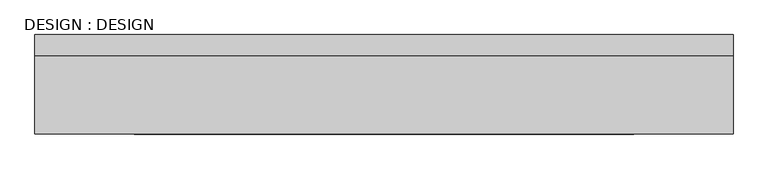
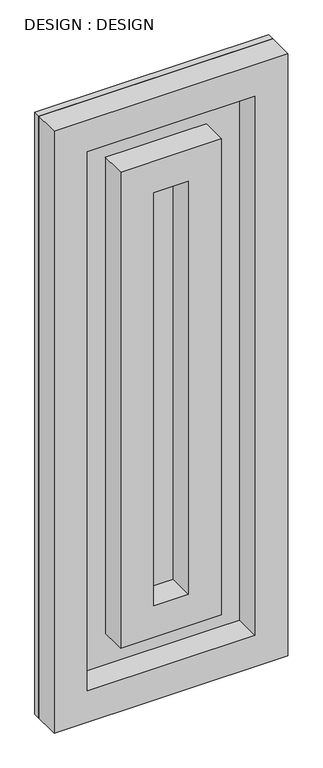
"""IFC4 building model written with IfcOpenShell, lengths in millimetres: proxy geometry, DESIGN : DESIGN."""

from ifc_helpers import new_model, si_unit, frame, origin, origin_with_axes, place, context, project, spatial, polyline, outline, extrude, source, transform, mapped, element, save


def design_design_9549e9b3(model_context):
    return source(origin(), model_context, "Body", "SweptSolid", [
        extrude(outline(polyline([(-3101.9879317, -6074.6691574), (-5245.26735, -6074.6691574), (-5245.26735, -6010.8688563), (-3101.9879317, -6010.8688563), (-3101.9879317, -6074.6691574)])), origin_with_axes(), (0.0, 0.0, 1.0), 5834.5767793),
        extrude(outline(polyline([(0.0, -3101.9879317), (5834.5767793, -3101.9879317), (5834.5767793, -5245.26735), (0.0, -5245.26735), (0.0, -3101.9879317)]), holes=[polyline([(5529.7767793, -3406.7879317), (304.8, -3406.7879317), (304.8, -4940.46735), (5529.7767793, -4940.46735), (5529.7767793, -3406.7879317)])]), frame((0.0, -6315.6688563, 0.0), z_axis=(0.0, 1.0, 0.0), x_axis=(0.0, 0.0, 1.0)), (0.0, 0.0, 1.0), 304.8),
        extrude(outline(polyline([(5224.9767793, -3711.5879317), (5224.9767793, -4635.66735), (609.6, -4635.66735), (609.6, -3711.5879317), (5224.9767793, -3711.5879317)]), holes=[polyline([(4920.1767793, -4016.3879317), (914.4, -4016.3879317), (914.4, -4330.86735), (4920.1767793, -4330.86735), (4920.1767793, -4016.3879317)])]), frame((0.0, -6315.6688563, 0.0), z_axis=(0.0, 1.0, 0.0), x_axis=(0.0, 0.0, 1.0)), (0.0, 0.0, 1.0), 304.8),
    ])


if __name__ == "__main__":
    model = new_model("IFC4")
    model_context = context("Model", 3, world=origin())
    ifc_project = project(units=[si_unit("LENGTHUNIT", "METRE", prefix="MILLI")], contexts=[model_context])
    site = spatial("IfcSite", under=ifc_project)
    building = spatial("IfcBuilding", under=site)
    placement = place(None, origin())
    design_design_shape = design_design_9549e9b3(model_context)
    element("IfcBuildingElementProxy", 1, Name="DESIGN : DESIGN", ObjectType="DESIGN : DESIGN", at=placement, inside=building, context=model_context, shape_type="MappedRepresentation", body=[
        mapped(design_design_shape, transform((0.0, 0.0, 0.0), x_axis=(1.0, 0.0, 0.0), y_axis=(0.0, 1.0, 0.0), z_axis=(0.0, 0.0, 1.0))),
    ])
    save(model, "model.ifc")

# Revit data of these elements
# Element 1 (IfcBuildingElementProxy, "DESIGN : DESIGN")
#   Materials on its faces: "PAINT 1", "Wood Planks"
# Materials
#   "PAINT 1": class "Generic", colour RGB 120 120 120, transparency 0, Cost = 0
#   "Wood Planks": class "Wood", colour RGB 193 160 115, transparency 0, Description = "Physical material.", Cost = 0
